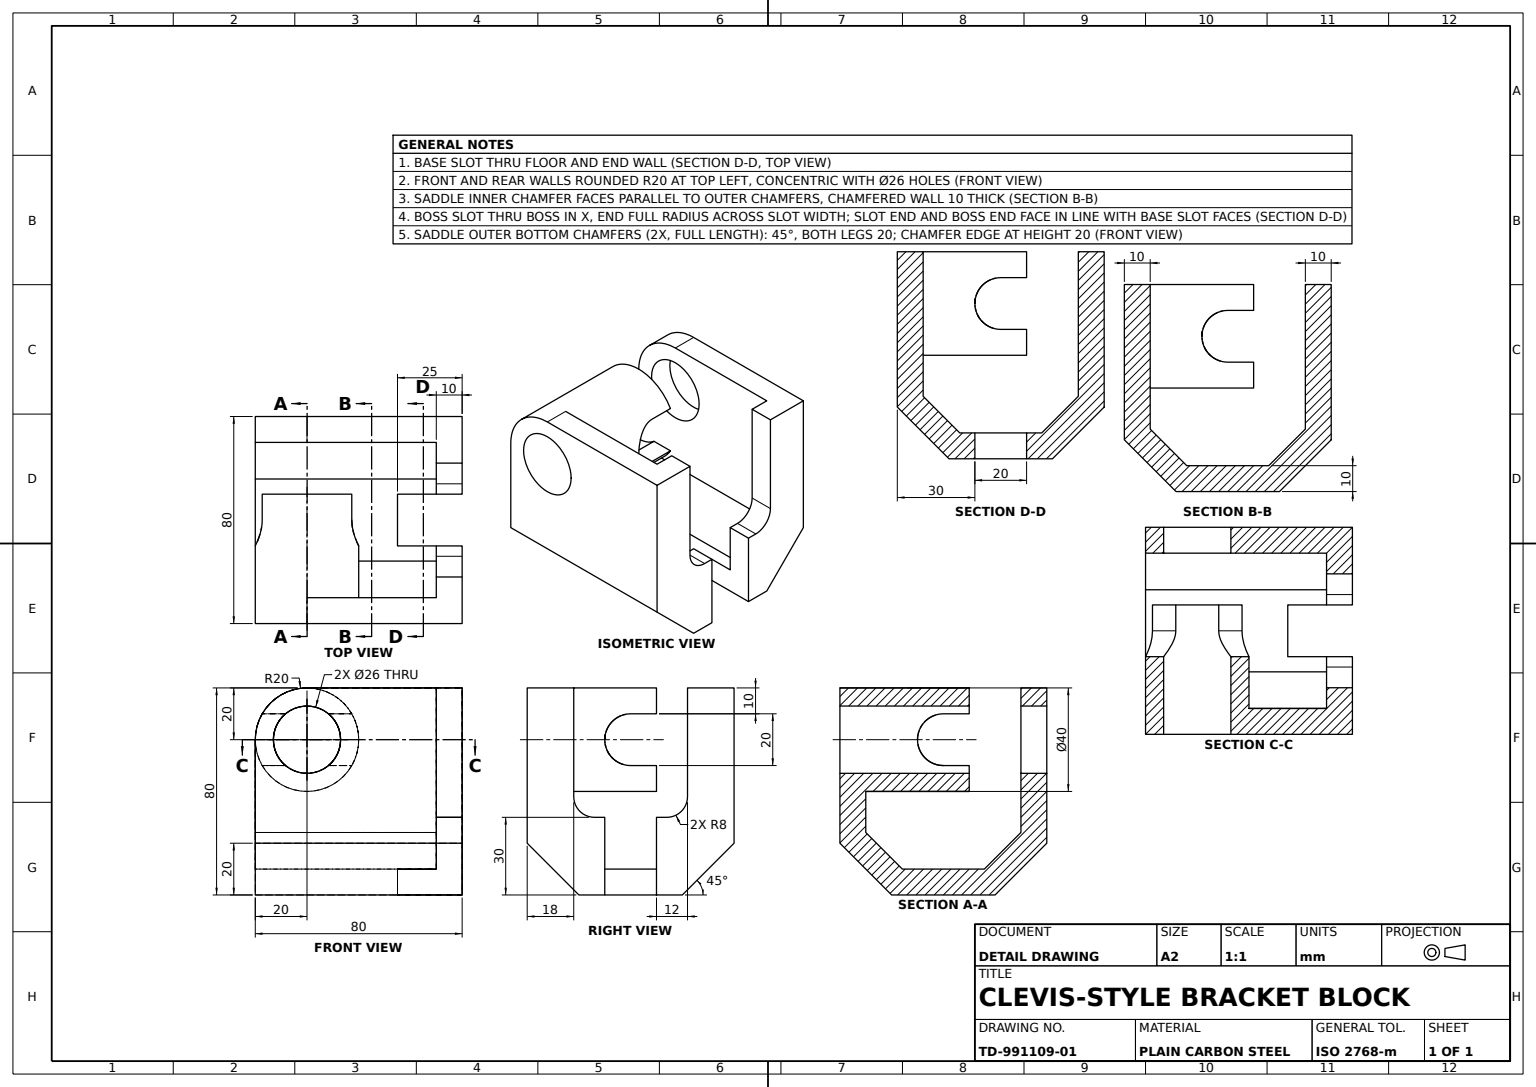
SolidWorks part; units mm, degrees
material "Plain Carbon Steel"
ref_plane "Front Plane" through (0, 0, 0) normal (0, 0, 1) x (1, 0, 0)
ref_plane "Top Plane" through (0, 0, 0) normal (0, 1, 0) x (1, 0, 0)
ref_plane "Right Plane" through (0, 0, 0) normal (1, 0, 0) x (0, 0, -1)
sketch "Saddle Profile Sketch" plane through (0, 0, 0) normal (1, 0, 0) x (0, 0, -1)
  line L0 (-20, 0) -> (20, 0)
  line L1 (20, 0) -> (40, 20)
  line L2 (40, 20) -> (40, 80)
  line L3 (40, 80) -> (30, 80)
  line L4 (30, 80) -> (30, 24.1421)
  line L5 (30, 24.1421) -> (15.8579, 10)
  line L6 (15.8579, 10) -> (-15.8579, 10)
  line L7 (0, 0) -> (0, 40.0304) construction
  line L8 (-30, 24.1421) -> (-15.8579, 10)
  line L9 (-30, 80) -> (-30, 24.1421)
  line L10 (-40, 80) -> (-30, 80)
  line L11 (-40, 20) -> (-40, 80)
  line L12 (-20, 0) -> (-40, 20)
  point P11 (0, 10)
  dimension "D1" = 20
  dimension "D2" = 20
  dimension "D3" = 80
  dimension "D4" = 80
  dimension "D5" = 10
  dimension "D6" = 10
  dimension "D7" = 10
extrude "Saddle Body" add sketch "Saddle Profile Sketch" along normal mid plane 80
fillet "Arm Top Rounds R20" radius 20 2 edges at (-40, 80, -35) (-40, 80, 35)
sketch "Side Boss Sketch" plane through (40, 0, 0) normal (1, 0, 0) x (0, 0, -1)
  line L0 (-30, 80) -> (-22, 80)
  line L1 (-22, 80) -> (-22, 38)
  line L2 (-14, 30) -> (-10, 30)
  line L3 (-10, 30) -> (-10, 10)
  line L4 (-20, 0) -> (20, 0) construction
  line L5 (0, 0) -> (0, 21.2573) construction
  line L6 (10, 30) -> (10, 10)
  line L7 (14, 30) -> (10, 30)
  line L8 (22, 80) -> (22, 38)
  line L9 (30, 80) -> (22, 80)
  line L10 (-30, 80) -> (-30, 24.1421)
  line L11 (-30, 24.1421) -> (-15.8579, 10)
  line L12 (-15.8579, 10) -> (-10, 10)
  line L13 (15.8579, 10) -> (-15.8579, 10) construction
  line L14 (15.8579, 10) -> (10, 10)
  line L15 (30, 24.1421) -> (15.8579, 10)
  line L16 (30, 80) -> (30, 24.1421)
  line L17 (-40, 80) -> (-40, 20) construction
  arc A0 (-22, 38) -> (-14, 30) centre (-14, 38) ccw
  arc A1 (22, 38) -> (14, 30) centre (14, 38) cw
  dimension "D1" = 8
  dimension "D2" = 18
  dimension "D3" = 20
  dimension "D4" = 30
extrude "Side Boss" add sketch "Side Boss Sketch" against normal blind 10
sketch "Boss Pocket Sketch" plane through (40, 0, 0) normal (1, 0, 0) x (0, 0, -1)
  line L0 (-20, 0) -> (20, 0) construction
  line L1 (-10, 10) -> (10, 10)
  line L2 (-10, 10) -> (-10, 0)
  line L3 (-10, 0) -> (10, 0)
  line L4 (10, 10) -> (10, 0)
  line L5 (10, 30) -> (10, 10) construction
extrude "Boss Pocket Cut" cut sketch "Boss Pocket Sketch" against normal blind 25
sketch "Journal Boss Sketch" plane through (0, 0, 30) normal (0, 0, -1) x (-1, 0, 0)
  circle A0 centre (20, 60) radius 20
  arc A1 (40, 60) -> (20, 80) centre (20, 60) ccw construction
extrude "Journal Boss" add sketch "Journal Boss Sketch" along normal blind 40
sketch "Base Slot Sketch" plane through (0, 0, 0) normal (1, 0, 0) x (0, 0, -1)
  line L0 (0, 70) -> (14.5313, 70)
  line L1 (14.5313, 70) -> (14.5313, 50)
  line L2 (14.5313, 50) -> (0, 50)
  arc A0 (0, 70) -> (0, 50) centre (0, 60) ccw
  dimension "D2" = 60
  dimension "D1" = 20
  dimension "D3" = 14.5313
extrude "Base Slot 20x60" cut sketch "Base Slot Sketch" against normal through all
sketch "Journal Bore Sketch" plane through (0, 0, -40) normal (0, 0, -1) x (-1, 0, 0)
  circle A0 centre (20, 60) radius 13
  arc A1 (40, 60) -> (20, 80) centre (20, 60) ccw construction
  dimension "D1" = 26
extrude "Journal Bore Ø26" cut sketch "Journal Bore Sketch" against normal through all
